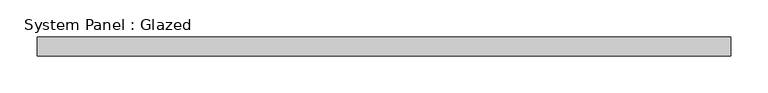
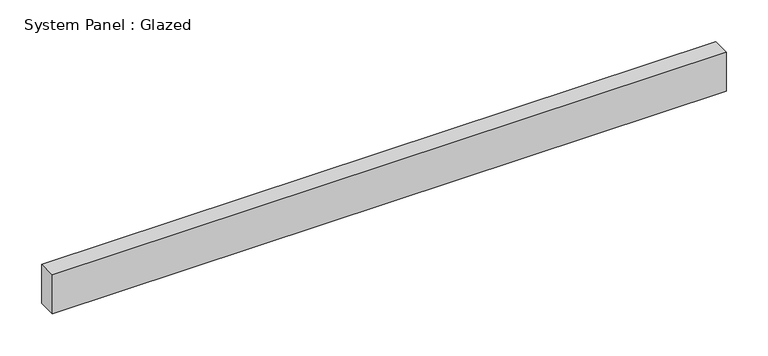
"""IFC4 building model written with IfcOpenShell, lengths in millimetres: plate geometry, System Panel : Glazed."""

from ifc_helpers import new_model, si_unit, origin, origin_with_axes, place, context, project, spatial, polyline, outline, extrude, source, transform, mapped, element, save


def system_panel_glazed_58efc156(model_context):
    return source(origin(), model_context, "Body", "SweptSolid", [
        extrude(outline(polyline([(467.0263558, 19.05), (-467.0263558, 19.05), (-467.0263558, 44.45), (467.0263558, 44.45), (467.0263558, 19.05)])), origin_with_axes(), (0.0, 0.0, 1.0), 57.15),
    ])


if __name__ == "__main__":
    model = new_model("IFC4")
    model_context = context("Model", 3, world=origin())
    ifc_project = project(units=[si_unit("LENGTHUNIT", "METRE", prefix="MILLI")], contexts=[model_context])
    site = spatial("IfcSite", under=ifc_project)
    building = spatial("IfcBuilding", under=site)
    placement = place(None, origin())
    system_panel_glazed_shape = system_panel_glazed_58efc156(model_context)
    element("IfcPlate", 1, ObjectType="System Panel : Glazed", at=placement, inside=building, context=model_context, shape_type="MappedRepresentation", body=[
        mapped(system_panel_glazed_shape, transform((0.0, 0.0, 0.0), x_axis=(1.0, 0.0, 0.0), y_axis=(0.0, 1.0, 0.0), z_axis=(0.0, 0.0, 1.0))),
    ])
    save(model, "model.ifc")

# Revit data of these elements
# Type "System Panel : Glazed"
#   Construction Type Id = "GSP4R"
#   Analytic Construction = "1/8 in Pilkington single glazing"
#   Visual Light Transmittance = 0.9
#   Solar Heat Gain Coefficient = 0.86
#   Heat Transfer Coefficient (U) = 1.18115 BTU/(h·ft²·°F)
#   Define Thermal Properties by = 1
# Element 1 (IfcPlate, "System Panel : Glazed")
#   Materials on its faces: "Glass"
# Materials
#   "Glass": class "Glass", colour RGB 0 128 192, transparency 0.75, Description = "Soda Lime Glass", Cost = 0
